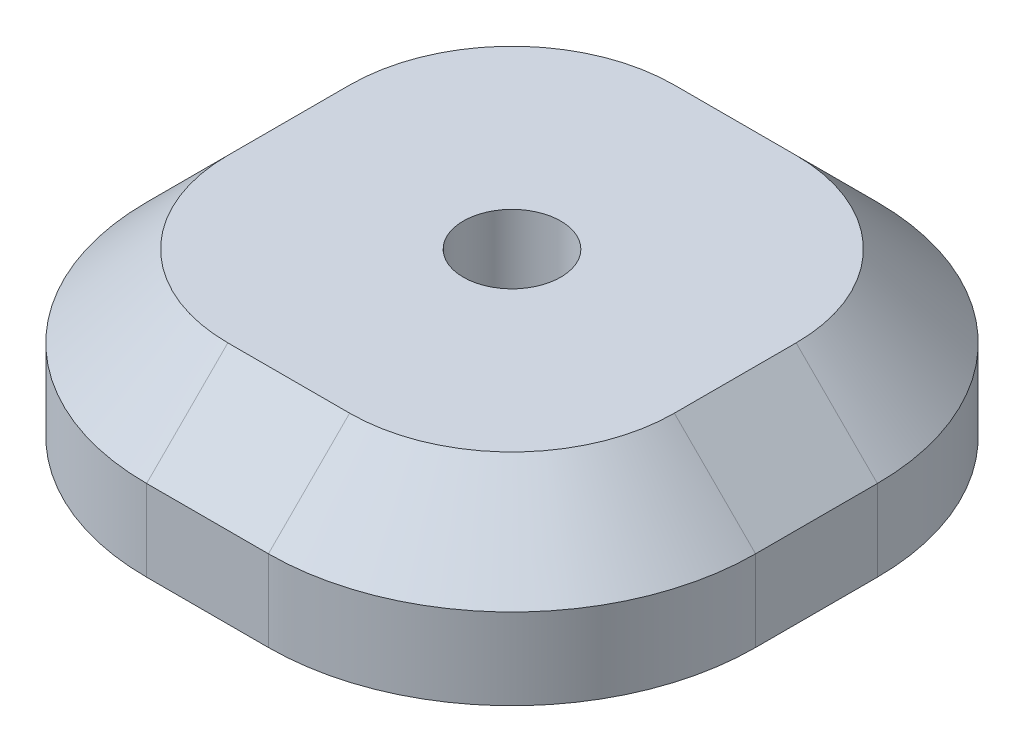
ISO-10303-21;
HEADER;
FILE_DESCRIPTION(('STEP AP214'),'2;1');
FILE_NAME('part.step','',(''),(''),'','','');
FILE_SCHEMA(('AUTOMOTIVE_DESIGN { 1 0 10303 214 1 1 1 1 }'));
ENDSEC;
DATA;
#1=APPLICATION_CONTEXT('core data for automotive mechanical design processes');
#2=APPLICATION_PROTOCOL_DEFINITION('international standard','automotive_design',2000,#1);
#3=PRODUCT_CONTEXT('',#1,'mechanical');
#4=PRODUCT('Part','Part','',(#3));
#5=PRODUCT_RELATED_PRODUCT_CATEGORY('part','',(#4));
#6=PRODUCT_DEFINITION_FORMATION('','',#4);
#7=PRODUCT_DEFINITION_CONTEXT('part definition',#1,'design');
#8=PRODUCT_DEFINITION('design','',#6,#7);
#9=PRODUCT_DEFINITION_SHAPE('','',#8);
#10=(LENGTH_UNIT() NAMED_UNIT(*) SI_UNIT(.MILLI.,.METRE.));
#11=(NAMED_UNIT(*) PLANE_ANGLE_UNIT() SI_UNIT($,.RADIAN.));
#12=(NAMED_UNIT(*) SI_UNIT($,.STERADIAN.) SOLID_ANGLE_UNIT());
#13=UNCERTAINTY_MEASURE_WITH_UNIT(LENGTH_MEASURE(1.E-05),#10,'distance_accuracy_value','');
#14=(GEOMETRIC_REPRESENTATION_CONTEXT(3) GLOBAL_UNCERTAINTY_ASSIGNED_CONTEXT((#13)) GLOBAL_UNIT_ASSIGNED_CONTEXT((#10,
#11,#12)) REPRESENTATION_CONTEXT('',''));
#15=CARTESIAN_POINT('',(0.,0.,0.));
#16=DIRECTION('',(0.,0.,1.));
#17=DIRECTION('',(1.,0.,0.));
#18=AXIS2_PLACEMENT_3D('',#15,#16,#17);
#19=CARTESIAN_POINT('',(37.5,20.,37.5));
#20=DIRECTION('',(-1.,0.,0.));
#21=DIRECTION('',(0.,0.,1.));
#22=AXIS2_PLACEMENT_3D('',#19,#20,#21);
#23=PLANE('',#22);
#24=DIRECTION('',(0.,-1.,0.));
#25=VECTOR('',#24,1.);
#26=CARTESIAN_POINT('',(37.5,20.,-7.5));
#27=LINE('',#26,#25);
#28=CARTESIAN_POINT('',(37.5,0.,-7.5));
#29=VERTEX_POINT('',#28);
#30=CARTESIAN_POINT('',(37.5,9.99999999999995,-7.5));
#31=VERTEX_POINT('',#30);
#32=EDGE_CURVE('E220',#29,#31,#27,.F.);
#33=ORIENTED_EDGE('',*,*,#32,.T.);
#34=DIRECTION('',(0.,0.,1.));
#35=VECTOR('',#34,1.);
#36=CARTESIAN_POINT('',(37.5,9.99999999999995,37.5));
#37=LINE('',#36,#35);
#38=CARTESIAN_POINT('',(37.5,9.99999999999995,7.5));
#39=VERTEX_POINT('',#38);
#40=EDGE_CURVE('E247',#31,#39,#37,.T.);
#41=ORIENTED_EDGE('',*,*,#40,.T.);
#42=DIRECTION('',(0.,-1.,0.));
#43=VECTOR('',#42,1.);
#44=CARTESIAN_POINT('',(37.5,20.,7.5));
#45=LINE('',#44,#43);
#46=CARTESIAN_POINT('',(37.5,0.,7.5));
#47=VERTEX_POINT('',#46);
#48=EDGE_CURVE('E214',#39,#47,#45,.T.);
#49=ORIENTED_EDGE('',*,*,#48,.T.);
#50=DIRECTION('',(0.,0.,-1.));
#51=VECTOR('',#50,1.);
#52=CARTESIAN_POINT('',(37.5,0.,37.5));
#53=LINE('',#52,#51);
#54=EDGE_CURVE('E183',#47,#29,#53,.T.);
#55=ORIENTED_EDGE('',*,*,#54,.T.);
#56=EDGE_LOOP('',(#33,#41,#49,#55));
#57=FACE_BOUND('',#56,.T.);
#58=ADVANCED_FACE('F41',(#57),#23,.F.);
#59=CARTESIAN_POINT('',(-37.5,20.,-37.5));
#60=DIRECTION('',(0.,0.,1.));
#61=DIRECTION('',(1.,0.,0.));
#62=AXIS2_PLACEMENT_3D('',#59,#60,#61);
#63=PLANE('',#62);
#64=DIRECTION('',(0.,-1.,0.));
#65=VECTOR('',#64,1.);
#66=CARTESIAN_POINT('',(-7.49999999999999,20.,-37.5));
#67=LINE('',#66,#65);
#68=CARTESIAN_POINT('',(-7.49999999999999,0.,-37.5));
#69=VERTEX_POINT('',#68);
#70=CARTESIAN_POINT('',(-7.49999999999999,9.99999999999995,-37.5));
#71=VERTEX_POINT('',#70);
#72=EDGE_CURVE('E215',#69,#71,#67,.F.);
#73=ORIENTED_EDGE('',*,*,#72,.T.);
#74=DIRECTION('',(1.,0.,0.));
#75=VECTOR('',#74,1.);
#76=CARTESIAN_POINT('',(-37.5,9.99999999999995,-37.5));
#77=LINE('',#76,#75);
#78=CARTESIAN_POINT('',(7.50000000000001,9.99999999999995,-37.5));
#79=VERTEX_POINT('',#78);
#80=EDGE_CURVE('E243',#71,#79,#77,.T.);
#81=ORIENTED_EDGE('',*,*,#80,.T.);
#82=DIRECTION('',(0.,-1.,0.));
#83=VECTOR('',#82,1.);
#84=CARTESIAN_POINT('',(7.50000000000001,20.,-37.5));
#85=LINE('',#84,#83);
#86=CARTESIAN_POINT('',(7.50000000000001,0.,-37.5));
#87=VERTEX_POINT('',#86);
#88=EDGE_CURVE('E209',#79,#87,#85,.T.);
#89=ORIENTED_EDGE('',*,*,#88,.T.);
#90=DIRECTION('',(-1.,0.,0.));
#91=VECTOR('',#90,1.);
#92=CARTESIAN_POINT('',(-37.5,0.,-37.5));
#93=LINE('',#92,#91);
#94=EDGE_CURVE('E186',#87,#69,#93,.T.);
#95=ORIENTED_EDGE('',*,*,#94,.T.);
#96=EDGE_LOOP('',(#73,#81,#89,#95));
#97=FACE_BOUND('',#96,.T.);
#98=ADVANCED_FACE('F317',(#97),#63,.F.);
#99=CARTESIAN_POINT('',(-37.5,20.,37.5));
#100=DIRECTION('',(1.,0.,0.));
#101=DIRECTION('',(0.,0.,-1.));
#102=AXIS2_PLACEMENT_3D('',#99,#100,#101);
#103=PLANE('',#102);
#104=DIRECTION('',(0.,-1.,0.));
#105=VECTOR('',#104,1.);
#106=CARTESIAN_POINT('',(-37.5,20.,7.5));
#107=LINE('',#106,#105);
#108=CARTESIAN_POINT('',(-37.5,0.,7.5));
#109=VERTEX_POINT('',#108);
#110=CARTESIAN_POINT('',(-37.5,9.99999999999995,7.5));
#111=VERTEX_POINT('',#110);
#112=EDGE_CURVE('E197',#109,#111,#107,.F.);
#113=ORIENTED_EDGE('',*,*,#112,.T.);
#114=DIRECTION('',(0.,0.,-1.));
#115=VECTOR('',#114,1.);
#116=CARTESIAN_POINT('',(-37.5,9.99999999999995,37.5));
#117=LINE('',#116,#115);
#118=CARTESIAN_POINT('',(-37.5,9.99999999999995,-7.5));
#119=VERTEX_POINT('',#118);
#120=EDGE_CURVE('E246',#111,#119,#117,.T.);
#121=ORIENTED_EDGE('',*,*,#120,.T.);
#122=DIRECTION('',(0.,-1.,0.));
#123=VECTOR('',#122,1.);
#124=CARTESIAN_POINT('',(-37.5,20.,-7.5));
#125=LINE('',#124,#123);
#126=CARTESIAN_POINT('',(-37.5,0.,-7.5));
#127=VERTEX_POINT('',#126);
#128=EDGE_CURVE('E199',#119,#127,#125,.T.);
#129=ORIENTED_EDGE('',*,*,#128,.T.);
#130=DIRECTION('',(0.,0.,1.));
#131=VECTOR('',#130,1.);
#132=CARTESIAN_POINT('',(-37.5,0.,37.5));
#133=LINE('',#132,#131);
#134=EDGE_CURVE('E193',#127,#109,#133,.T.);
#135=ORIENTED_EDGE('',*,*,#134,.T.);
#136=EDGE_LOOP('',(#113,#121,#129,#135));
#137=FACE_BOUND('',#136,.T.);
#138=ADVANCED_FACE('F292',(#137),#103,.F.);
#139=CARTESIAN_POINT('',(-37.5,20.,37.5));
#140=DIRECTION('',(0.,0.,-1.));
#141=DIRECTION('',(-1.,0.,0.));
#142=AXIS2_PLACEMENT_3D('',#139,#140,#141);
#143=PLANE('',#142);
#144=DIRECTION('',(0.,-1.,0.));
#145=VECTOR('',#144,1.);
#146=CARTESIAN_POINT('',(7.50000000000001,20.,37.5));
#147=LINE('',#146,#145);
#148=CARTESIAN_POINT('',(7.50000000000001,0.,37.5));
#149=VERTEX_POINT('',#148);
#150=CARTESIAN_POINT('',(7.50000000000001,9.99999999999995,37.5));
#151=VERTEX_POINT('',#150);
#152=EDGE_CURVE('E225',#149,#151,#147,.F.);
#153=ORIENTED_EDGE('',*,*,#152,.T.);
#154=DIRECTION('',(-1.,0.,0.));
#155=VECTOR('',#154,1.);
#156=CARTESIAN_POINT('',(-37.5,9.99999999999995,37.5));
#157=LINE('',#156,#155);
#158=CARTESIAN_POINT('',(-7.49999999999999,9.99999999999995,37.5));
#159=VERTEX_POINT('',#158);
#160=EDGE_CURVE('E11',#151,#159,#157,.T.);
#161=ORIENTED_EDGE('',*,*,#160,.T.);
#162=DIRECTION('',(0.,-1.,0.));
#163=VECTOR('',#162,1.);
#164=CARTESIAN_POINT('',(-7.49999999999999,20.,37.5));
#165=LINE('',#164,#163);
#166=CARTESIAN_POINT('',(-7.49999999999999,0.,37.5));
#167=VERTEX_POINT('',#166);
#168=EDGE_CURVE('E219',#159,#167,#165,.T.);
#169=ORIENTED_EDGE('',*,*,#168,.T.);
#170=DIRECTION('',(1.,0.,0.));
#171=VECTOR('',#170,1.);
#172=CARTESIAN_POINT('',(-37.5,0.,37.5));
#173=LINE('',#172,#171);
#174=EDGE_CURVE('E194',#167,#149,#173,.T.);
#175=ORIENTED_EDGE('',*,*,#174,.T.);
#176=EDGE_LOOP('',(#153,#161,#169,#175));
#177=FACE_BOUND('',#176,.T.);
#178=ADVANCED_FACE('F303',(#177),#143,.F.);
#179=CARTESIAN_POINT('',(0.,20.,0.));
#180=DIRECTION('',(0.,-1.,0.));
#181=DIRECTION('',(0.,0.,-1.));
#182=AXIS2_PLACEMENT_3D('',#179,#180,#181);
#183=PLANE('',#182);
#184=CARTESIAN_POINT('',(0.,20.,0.));
#185=DIRECTION('',(0.,1.,0.));
#186=DIRECTION('',(0.,0.,1.));
#187=AXIS2_PLACEMENT_3D('',#184,#185,#186);
#188=CIRCLE('',#187,5.99999999999999);
#189=CARTESIAN_POINT('',(0.,20.,5.99999999999999));
#190=VERTEX_POINT('',#189);
#191=EDGE_CURVE('E176',#190,#190,#188,.T.);
#192=ORIENTED_EDGE('',*,*,#191,.F.);
#193=EDGE_LOOP('',(#192));
#194=FACE_BOUND('',#193,.T.);
#195=CARTESIAN_POINT('',(7.50000000000001,20.,-7.5));
#196=DIRECTION('',(0.,-1.,0.));
#197=DIRECTION('',(0.,0.,-1.));
#198=AXIS2_PLACEMENT_3D('',#195,#196,#197);
#199=CIRCLE('',#198,20.);
#200=CARTESIAN_POINT('',(27.5,20.,-7.5));
#201=VERTEX_POINT('',#200);
#202=CARTESIAN_POINT('',(7.50000000000001,20.,-27.5));
#203=VERTEX_POINT('',#202);
#204=EDGE_CURVE('E234',#201,#203,#199,.F.);
#205=ORIENTED_EDGE('',*,*,#204,.T.);
#206=DIRECTION('',(-1.,0.,0.));
#207=VECTOR('',#206,1.);
#208=CARTESIAN_POINT('',(0.,20.,-27.5));
#209=LINE('',#208,#207);
#210=CARTESIAN_POINT('',(-7.49999999999999,20.,-27.5));
#211=VERTEX_POINT('',#210);
#212=EDGE_CURVE('E236',#203,#211,#209,.T.);
#213=ORIENTED_EDGE('',*,*,#212,.T.);
#214=CARTESIAN_POINT('',(-7.49999999999999,20.,-7.5));
#215=DIRECTION('',(0.,-1.,0.));
#216=DIRECTION('',(0.,0.,-1.));
#217=AXIS2_PLACEMENT_3D('',#214,#215,#216);
#218=CIRCLE('',#217,20.);
#219=CARTESIAN_POINT('',(-27.5,20.,-7.5));
#220=VERTEX_POINT('',#219);
#221=EDGE_CURVE('E237',#211,#220,#218,.F.);
#222=ORIENTED_EDGE('',*,*,#221,.T.);
#223=DIRECTION('',(0.,0.,1.));
#224=VECTOR('',#223,1.);
#225=CARTESIAN_POINT('',(-27.5,20.,0.));
#226=LINE('',#225,#224);
#227=CARTESIAN_POINT('',(-27.5,20.,7.5));
#228=VERTEX_POINT('',#227);
#229=EDGE_CURVE('E235',#220,#228,#226,.T.);
#230=ORIENTED_EDGE('',*,*,#229,.T.);
#231=CARTESIAN_POINT('',(-7.49999999999999,20.,7.5));
#232=DIRECTION('',(0.,-1.,0.));
#233=DIRECTION('',(0.,0.,-1.));
#234=AXIS2_PLACEMENT_3D('',#231,#232,#233);
#235=CIRCLE('',#234,20.);
#236=CARTESIAN_POINT('',(-7.49999999999999,20.,27.5));
#237=VERTEX_POINT('',#236);
#238=EDGE_CURVE('E226',#228,#237,#235,.F.);
#239=ORIENTED_EDGE('',*,*,#238,.T.);
#240=DIRECTION('',(1.,0.,0.));
#241=VECTOR('',#240,1.);
#242=CARTESIAN_POINT('',(0.,20.,27.5));
#243=LINE('',#242,#241);
#244=CARTESIAN_POINT('',(7.50000000000001,20.,27.5));
#245=VERTEX_POINT('',#244);
#246=EDGE_CURVE('E221',#237,#245,#243,.T.);
#247=ORIENTED_EDGE('',*,*,#246,.T.);
#248=CARTESIAN_POINT('',(7.50000000000001,20.,7.5));
#249=DIRECTION('',(0.,-1.,0.));
#250=DIRECTION('',(0.,0.,-1.));
#251=AXIS2_PLACEMENT_3D('',#248,#249,#250);
#252=CIRCLE('',#251,20.);
#253=CARTESIAN_POINT('',(27.5,20.,7.5));
#254=VERTEX_POINT('',#253);
#255=EDGE_CURVE('E228',#245,#254,#252,.F.);
#256=ORIENTED_EDGE('',*,*,#255,.T.);
#257=DIRECTION('',(0.,0.,-1.));
#258=VECTOR('',#257,1.);
#259=CARTESIAN_POINT('',(27.5,20.,0.));
#260=LINE('',#259,#258);
#261=EDGE_CURVE('E229',#254,#201,#260,.T.);
#262=ORIENTED_EDGE('',*,*,#261,.T.);
#263=EDGE_LOOP('',(#205,#213,#222,#230,#239,#247,#256,#262));
#264=FACE_BOUND('',#263,.T.);
#265=ADVANCED_FACE('F332',(#194,#264),#183,.F.);
#266=CARTESIAN_POINT('',(0.,0.,0.));
#267=DIRECTION('',(0.,-1.,0.));
#268=DIRECTION('',(0.,0.,-1.));
#269=AXIS2_PLACEMENT_3D('',#266,#267,#268);
#270=PLANE('',#269);
#271=CARTESIAN_POINT('',(-12.5,0.,12.5));
#272=DIRECTION('',(0.,-1.,0.));
#273=DIRECTION('',(0.,0.,-1.));
#274=AXIS2_PLACEMENT_3D('',#271,#272,#273);
#275=CIRCLE('',#274,5.99999999999999);
#276=CARTESIAN_POINT('',(-12.5,0.,6.50000000000001));
#277=VERTEX_POINT('',#276);
#278=EDGE_CURVE('E156',#277,#277,#275,.T.);
#279=ORIENTED_EDGE('',*,*,#278,.F.);
#280=EDGE_LOOP('',(#279));
#281=FACE_BOUND('',#280,.T.);
#282=CARTESIAN_POINT('',(12.5,0.,12.5));
#283=DIRECTION('',(0.,-1.,0.));
#284=DIRECTION('',(0.,0.,-1.));
#285=AXIS2_PLACEMENT_3D('',#282,#283,#284);
#286=CIRCLE('',#285,5.99999999999999);
#287=CARTESIAN_POINT('',(12.5,0.,6.50000000000001));
#288=VERTEX_POINT('',#287);
#289=EDGE_CURVE('E154',#288,#288,#286,.T.);
#290=ORIENTED_EDGE('',*,*,#289,.F.);
#291=EDGE_LOOP('',(#290));
#292=FACE_BOUND('',#291,.T.);
#293=CARTESIAN_POINT('',(12.5,0.,-12.5));
#294=DIRECTION('',(0.,-1.,0.));
#295=DIRECTION('',(0.,0.,-1.));
#296=AXIS2_PLACEMENT_3D('',#293,#294,#295);
#297=CIRCLE('',#296,5.99999999999999);
#298=CARTESIAN_POINT('',(12.5,0.,-18.5));
#299=VERTEX_POINT('',#298);
#300=EDGE_CURVE('E167',#299,#299,#297,.T.);
#301=ORIENTED_EDGE('',*,*,#300,.F.);
#302=EDGE_LOOP('',(#301));
#303=FACE_BOUND('',#302,.T.);
#304=CARTESIAN_POINT('',(-12.5,0.,-12.5));
#305=DIRECTION('',(0.,-1.,0.));
#306=DIRECTION('',(0.,0.,-1.));
#307=AXIS2_PLACEMENT_3D('',#304,#305,#306);
#308=CIRCLE('',#307,5.99999999999999);
#309=CARTESIAN_POINT('',(-12.5,0.,-18.5));
#310=VERTEX_POINT('',#309);
#311=EDGE_CURVE('E175',#310,#310,#308,.T.);
#312=ORIENTED_EDGE('',*,*,#311,.F.);
#313=EDGE_LOOP('',(#312));
#314=FACE_BOUND('',#313,.T.);
#315=ORIENTED_EDGE('',*,*,#134,.F.);
#316=CARTESIAN_POINT('',(-7.49999999999999,0.,-7.5));
#317=DIRECTION('',(0.,-1.,0.));
#318=DIRECTION('',(0.,0.,-1.));
#319=AXIS2_PLACEMENT_3D('',#316,#317,#318);
#320=CIRCLE('',#319,30.);
#321=EDGE_CURVE('E208',#127,#69,#320,.T.);
#322=ORIENTED_EDGE('',*,*,#321,.T.);
#323=ORIENTED_EDGE('',*,*,#94,.F.);
#324=CARTESIAN_POINT('',(7.50000000000001,0.,-7.5));
#325=DIRECTION('',(0.,-1.,0.));
#326=DIRECTION('',(0.,0.,-1.));
#327=AXIS2_PLACEMENT_3D('',#324,#325,#326);
#328=CIRCLE('',#327,30.);
#329=EDGE_CURVE('E206',#87,#29,#328,.T.);
#330=ORIENTED_EDGE('',*,*,#329,.T.);
#331=ORIENTED_EDGE('',*,*,#54,.F.);
#332=CARTESIAN_POINT('',(7.50000000000001,0.,7.5));
#333=DIRECTION('',(0.,-1.,0.));
#334=DIRECTION('',(0.,0.,-1.));
#335=AXIS2_PLACEMENT_3D('',#332,#333,#334);
#336=CIRCLE('',#335,30.);
#337=EDGE_CURVE('E204',#47,#149,#336,.T.);
#338=ORIENTED_EDGE('',*,*,#337,.T.);
#339=ORIENTED_EDGE('',*,*,#174,.F.);
#340=CARTESIAN_POINT('',(-7.49999999999999,0.,7.5));
#341=DIRECTION('',(0.,-1.,0.));
#342=DIRECTION('',(0.,0.,-1.));
#343=AXIS2_PLACEMENT_3D('',#340,#341,#342);
#344=CIRCLE('',#343,30.);
#345=EDGE_CURVE('E205',#167,#109,#344,.T.);
#346=ORIENTED_EDGE('',*,*,#345,.T.);
#347=EDGE_LOOP('',(#315,#322,#323,#330,#331,#338,#339,#346));
#348=FACE_BOUND('',#347,.T.);
#349=ADVANCED_FACE('F298',(#281,#292,#303,#314,#348),#270,.T.);
#350=CARTESIAN_POINT('',(-7.49999999999999,20.,-7.5));
#351=DIRECTION('',(0.,-1.,0.));
#352=DIRECTION('',(0.,0.,-1.));
#353=AXIS2_PLACEMENT_3D('',#350,#351,#352);
#354=CYLINDRICAL_SURFACE('',#353,30.);
#355=ORIENTED_EDGE('',*,*,#128,.F.);
#356=CARTESIAN_POINT('',(-7.49999999999999,9.99999999999995,-7.5));
#357=DIRECTION('',(0.,-1.,0.));
#358=DIRECTION('',(0.,0.,-1.));
#359=AXIS2_PLACEMENT_3D('',#356,#357,#358);
#360=CIRCLE('',#359,30.);
#361=EDGE_CURVE('E242',#119,#71,#360,.T.);
#362=ORIENTED_EDGE('',*,*,#361,.T.);
#363=ORIENTED_EDGE('',*,*,#72,.F.);
#364=ORIENTED_EDGE('',*,*,#321,.F.);
#365=EDGE_LOOP('',(#355,#362,#363,#364));
#366=FACE_BOUND('',#365,.T.);
#367=ADVANCED_FACE('F352',(#366),#354,.T.);
#368=CARTESIAN_POINT('',(7.50000000000001,20.,-7.5));
#369=DIRECTION('',(0.,-1.,0.));
#370=DIRECTION('',(0.,0.,-1.));
#371=AXIS2_PLACEMENT_3D('',#368,#369,#370);
#372=CYLINDRICAL_SURFACE('',#371,30.);
#373=ORIENTED_EDGE('',*,*,#88,.F.);
#374=CARTESIAN_POINT('',(7.50000000000001,9.99999999999995,-7.5));
#375=DIRECTION('',(0.,-1.,0.));
#376=DIRECTION('',(0.,0.,-1.));
#377=AXIS2_PLACEMENT_3D('',#374,#375,#376);
#378=CIRCLE('',#377,30.);
#379=EDGE_CURVE('E248',#79,#31,#378,.T.);
#380=ORIENTED_EDGE('',*,*,#379,.T.);
#381=ORIENTED_EDGE('',*,*,#32,.F.);
#382=ORIENTED_EDGE('',*,*,#329,.F.);
#383=EDGE_LOOP('',(#373,#380,#381,#382));
#384=FACE_BOUND('',#383,.T.);
#385=ADVANCED_FACE('F310',(#384),#372,.T.);
#386=CARTESIAN_POINT('',(7.50000000000001,20.,7.5));
#387=DIRECTION('',(0.,-1.,0.));
#388=DIRECTION('',(0.,0.,-1.));
#389=AXIS2_PLACEMENT_3D('',#386,#387,#388);
#390=CYLINDRICAL_SURFACE('',#389,30.);
#391=ORIENTED_EDGE('',*,*,#48,.F.);
#392=CARTESIAN_POINT('',(7.50000000000001,9.99999999999995,7.5));
#393=DIRECTION('',(0.,-1.,0.));
#394=DIRECTION('',(0.,0.,-1.));
#395=AXIS2_PLACEMENT_3D('',#392,#393,#394);
#396=CIRCLE('',#395,30.);
#397=EDGE_CURVE('E51',#39,#151,#396,.T.);
#398=ORIENTED_EDGE('',*,*,#397,.T.);
#399=ORIENTED_EDGE('',*,*,#152,.F.);
#400=ORIENTED_EDGE('',*,*,#337,.F.);
#401=EDGE_LOOP('',(#391,#398,#399,#400));
#402=FACE_BOUND('',#401,.T.);
#403=ADVANCED_FACE('F305',(#402),#390,.T.);
#404=CARTESIAN_POINT('',(-7.49999999999999,20.,7.5));
#405=DIRECTION('',(0.,-1.,0.));
#406=DIRECTION('',(0.,0.,-1.));
#407=AXIS2_PLACEMENT_3D('',#404,#405,#406);
#408=CYLINDRICAL_SURFACE('',#407,30.);
#409=ORIENTED_EDGE('',*,*,#168,.F.);
#410=CARTESIAN_POINT('',(-7.49999999999999,9.99999999999995,7.5));
#411=DIRECTION('',(0.,-1.,0.));
#412=DIRECTION('',(0.,0.,-1.));
#413=AXIS2_PLACEMENT_3D('',#410,#411,#412);
#414=CIRCLE('',#413,30.);
#415=EDGE_CURVE('E252',#159,#111,#414,.T.);
#416=ORIENTED_EDGE('',*,*,#415,.T.);
#417=ORIENTED_EDGE('',*,*,#112,.F.);
#418=ORIENTED_EDGE('',*,*,#345,.F.);
#419=EDGE_LOOP('',(#409,#416,#417,#418));
#420=FACE_BOUND('',#419,.T.);
#421=ADVANCED_FACE('F286',(#420),#408,.T.);
#422=CARTESIAN_POINT('',(0.,20.,27.5));
#423=DIRECTION('',(0.,-0.707106781186546,-0.707106781186549));
#424=DIRECTION('',(1.,0.,0.));
#425=AXIS2_PLACEMENT_3D('',#422,#423,#424);
#426=PLANE('',#425);
#427=DIRECTION('',(0.,0.707106781186549,-0.707106781186546));
#428=VECTOR('',#427,1.);
#429=CARTESIAN_POINT('',(-7.49999999999999,9.99999999999995,37.5));
#430=LINE('',#429,#428);
#431=EDGE_CURVE('E267',#159,#237,#430,.T.);
#432=ORIENTED_EDGE('',*,*,#431,.F.);
#433=ORIENTED_EDGE('',*,*,#160,.F.);
#434=DIRECTION('',(0.,-0.707106781186549,0.707106781186546));
#435=VECTOR('',#434,1.);
#436=CARTESIAN_POINT('',(7.50000000000001,20.,27.5));
#437=LINE('',#436,#435);
#438=EDGE_CURVE('E46',#245,#151,#437,.T.);
#439=ORIENTED_EDGE('',*,*,#438,.F.);
#440=ORIENTED_EDGE('',*,*,#246,.F.);
#441=EDGE_LOOP('',(#432,#433,#439,#440));
#442=FACE_BOUND('',#441,.T.);
#443=ADVANCED_FACE('F42',(#442),#426,.F.);
#444=CARTESIAN_POINT('',(7.50000000000001,20.,7.5));
#445=DIRECTION('',(0.,-1.,0.));
#446=DIRECTION('',(0.,0.,-1.));
#447=AXIS2_PLACEMENT_3D('',#444,#445,#446);
#448=CONICAL_SURFACE('',#447,20.,0.785398163397446);
#449=ORIENTED_EDGE('',*,*,#438,.T.);
#450=ORIENTED_EDGE('',*,*,#397,.F.);
#451=DIRECTION('',(0.707106781186546,-0.707106781186549,0.));
#452=VECTOR('',#451,1.);
#453=CARTESIAN_POINT('',(27.5,20.,7.5));
#454=LINE('',#453,#452);
#455=EDGE_CURVE('E270',#254,#39,#454,.T.);
#456=ORIENTED_EDGE('',*,*,#455,.F.);
#457=ORIENTED_EDGE('',*,*,#255,.F.);
#458=EDGE_LOOP('',(#449,#450,#456,#457));
#459=FACE_BOUND('',#458,.T.);
#460=ADVANCED_FACE('F276',(#459),#448,.T.);
#461=CARTESIAN_POINT('',(-7.49999999999999,20.,7.5));
#462=DIRECTION('',(0.,-1.,0.));
#463=DIRECTION('',(0.,0.,-1.));
#464=AXIS2_PLACEMENT_3D('',#461,#462,#463);
#465=CONICAL_SURFACE('',#464,20.,0.785398163397446);
#466=ORIENTED_EDGE('',*,*,#431,.T.);
#467=ORIENTED_EDGE('',*,*,#238,.F.);
#468=DIRECTION('',(0.707106781186546,0.707106781186549,0.));
#469=VECTOR('',#468,1.);
#470=CARTESIAN_POINT('',(-37.5,9.99999999999995,7.5));
#471=LINE('',#470,#469);
#472=EDGE_CURVE('E262',#111,#228,#471,.T.);
#473=ORIENTED_EDGE('',*,*,#472,.F.);
#474=ORIENTED_EDGE('',*,*,#415,.F.);
#475=EDGE_LOOP('',(#466,#467,#473,#474));
#476=FACE_BOUND('',#475,.T.);
#477=ADVANCED_FACE('F282',(#476),#465,.T.);
#478=CARTESIAN_POINT('',(27.5,20.,0.));
#479=DIRECTION('',(-0.707106781186549,-0.707106781186546,0.));
#480=DIRECTION('',(0.,0.,-1.));
#481=AXIS2_PLACEMENT_3D('',#478,#479,#480);
#482=PLANE('',#481);
#483=ORIENTED_EDGE('',*,*,#455,.T.);
#484=ORIENTED_EDGE('',*,*,#40,.F.);
#485=DIRECTION('',(0.707106781186546,-0.707106781186549,0.));
#486=VECTOR('',#485,1.);
#487=CARTESIAN_POINT('',(27.5,20.,-7.5));
#488=LINE('',#487,#486);
#489=EDGE_CURVE('E261',#201,#31,#488,.T.);
#490=ORIENTED_EDGE('',*,*,#489,.F.);
#491=ORIENTED_EDGE('',*,*,#261,.F.);
#492=EDGE_LOOP('',(#483,#484,#490,#491));
#493=FACE_BOUND('',#492,.T.);
#494=ADVANCED_FACE('F331',(#493),#482,.F.);
#495=CARTESIAN_POINT('',(-27.5,20.,0.));
#496=DIRECTION('',(0.707106781186549,-0.707106781186546,0.));
#497=DIRECTION('',(0.,0.,1.));
#498=AXIS2_PLACEMENT_3D('',#495,#496,#497);
#499=PLANE('',#498);
#500=ORIENTED_EDGE('',*,*,#472,.T.);
#501=ORIENTED_EDGE('',*,*,#229,.F.);
#502=DIRECTION('',(0.707106781186546,0.707106781186549,0.));
#503=VECTOR('',#502,1.);
#504=CARTESIAN_POINT('',(-37.5,9.99999999999995,-7.5));
#505=LINE('',#504,#503);
#506=EDGE_CURVE('E256',#119,#220,#505,.T.);
#507=ORIENTED_EDGE('',*,*,#506,.F.);
#508=ORIENTED_EDGE('',*,*,#120,.F.);
#509=EDGE_LOOP('',(#500,#501,#507,#508));
#510=FACE_BOUND('',#509,.T.);
#511=ADVANCED_FACE('F338',(#510),#499,.F.);
#512=CARTESIAN_POINT('',(7.50000000000001,20.,-7.5));
#513=DIRECTION('',(0.,-1.,0.));
#514=DIRECTION('',(0.,0.,-1.));
#515=AXIS2_PLACEMENT_3D('',#512,#513,#514);
#516=CONICAL_SURFACE('',#515,20.,0.785398163397446);
#517=ORIENTED_EDGE('',*,*,#489,.T.);
#518=ORIENTED_EDGE('',*,*,#379,.F.);
#519=DIRECTION('',(0.,-0.707106781186549,-0.707106781186546));
#520=VECTOR('',#519,1.);
#521=CARTESIAN_POINT('',(7.50000000000001,20.,-27.5));
#522=LINE('',#521,#520);
#523=EDGE_CURVE('E258',#203,#79,#522,.T.);
#524=ORIENTED_EDGE('',*,*,#523,.F.);
#525=ORIENTED_EDGE('',*,*,#204,.F.);
#526=EDGE_LOOP('',(#517,#518,#524,#525));
#527=FACE_BOUND('',#526,.T.);
#528=ADVANCED_FACE('F311',(#527),#516,.T.);
#529=CARTESIAN_POINT('',(-7.49999999999999,20.,-7.5));
#530=DIRECTION('',(0.,-1.,0.));
#531=DIRECTION('',(0.,0.,-1.));
#532=AXIS2_PLACEMENT_3D('',#529,#530,#531);
#533=CONICAL_SURFACE('',#532,20.,0.785398163397446);
#534=ORIENTED_EDGE('',*,*,#506,.T.);
#535=ORIENTED_EDGE('',*,*,#221,.F.);
#536=DIRECTION('',(0.,0.707106781186549,0.707106781186546));
#537=VECTOR('',#536,1.);
#538=CARTESIAN_POINT('',(-7.49999999999999,9.99999999999995,-37.5));
#539=LINE('',#538,#537);
#540=EDGE_CURVE('E184',#71,#211,#539,.T.);
#541=ORIENTED_EDGE('',*,*,#540,.F.);
#542=ORIENTED_EDGE('',*,*,#361,.F.);
#543=EDGE_LOOP('',(#534,#535,#541,#542));
#544=FACE_BOUND('',#543,.T.);
#545=ADVANCED_FACE('F330',(#544),#533,.T.);
#546=CARTESIAN_POINT('',(0.,20.,-27.5));
#547=DIRECTION('',(0.,-0.707106781186546,0.707106781186549));
#548=DIRECTION('',(-1.,0.,0.));
#549=AXIS2_PLACEMENT_3D('',#546,#547,#548);
#550=PLANE('',#549);
#551=ORIENTED_EDGE('',*,*,#523,.T.);
#552=ORIENTED_EDGE('',*,*,#80,.F.);
#553=ORIENTED_EDGE('',*,*,#540,.T.);
#554=ORIENTED_EDGE('',*,*,#212,.F.);
#555=EDGE_LOOP('',(#551,#552,#553,#554));
#556=FACE_BOUND('',#555,.T.);
#557=ADVANCED_FACE('F323',(#556),#550,.F.);
#558=CARTESIAN_POINT('',(0.,10.,0.));
#559=DIRECTION('',(0.,1.,0.));
#560=DIRECTION('',(0.,0.,1.));
#561=AXIS2_PLACEMENT_3D('',#558,#559,#560);
#562=CONICAL_SURFACE('',#561,5.99999999999999,1.02974425867665);
#563=CARTESIAN_POINT('',(0.,6.39483628583465,0.));
#564=VERTEX_POINT('',#563);
#565=VERTEX_LOOP('',#564);
#566=FACE_BOUND('',#565,.T.);
#567=CARTESIAN_POINT('',(0.,10.,0.));
#568=DIRECTION('',(0.,1.,0.));
#569=DIRECTION('',(0.,0.,1.));
#570=AXIS2_PLACEMENT_3D('',#567,#568,#569);
#571=CIRCLE('',#570,5.99999999999999);
#572=CARTESIAN_POINT('',(0.,10.,5.99999999999999));
#573=VERTEX_POINT('',#572);
#574=EDGE_CURVE('E182',#573,#573,#571,.T.);
#575=ORIENTED_EDGE('',*,*,#574,.T.);
#576=EDGE_LOOP('',(#575));
#577=FACE_BOUND('',#576,.T.);
#578=ADVANCED_FACE('F367',(#566,#577),#562,.F.);
#579=CARTESIAN_POINT('',(0.,20.,0.));
#580=DIRECTION('',(0.,1.,0.));
#581=DIRECTION('',(0.,0.,1.));
#582=AXIS2_PLACEMENT_3D('',#579,#580,#581);
#583=CYLINDRICAL_SURFACE('',#582,5.99999999999999);
#584=ORIENTED_EDGE('',*,*,#574,.F.);
#585=EDGE_LOOP('',(#584));
#586=FACE_BOUND('',#585,.T.);
#587=ORIENTED_EDGE('',*,*,#191,.T.);
#588=EDGE_LOOP('',(#587));
#589=FACE_BOUND('',#588,.T.);
#590=ADVANCED_FACE('F504',(#586,#589),#583,.F.);
#591=CARTESIAN_POINT('',(-12.5,9.99999999999999,-12.5));
#592=DIRECTION('',(0.,-1.,0.));
#593=DIRECTION('',(0.,0.,-1.));
#594=AXIS2_PLACEMENT_3D('',#591,#592,#593);
#595=CONICAL_SURFACE('',#594,5.99999999999999,1.02974425867665);
#596=CARTESIAN_POINT('',(-12.5,13.6051637141654,-12.5));
#597=VERTEX_POINT('',#596);
#598=VERTEX_LOOP('',#597);
#599=FACE_BOUND('',#598,.T.);
#600=CARTESIAN_POINT('',(-12.5,9.99999999999999,-12.5));
#601=DIRECTION('',(0.,-1.,0.));
#602=DIRECTION('',(0.,0.,-1.));
#603=AXIS2_PLACEMENT_3D('',#600,#601,#602);
#604=CIRCLE('',#603,5.99999999999999);
#605=CARTESIAN_POINT('',(-12.5,9.99999999999999,-18.5));
#606=VERTEX_POINT('',#605);
#607=EDGE_CURVE('E174',#606,#606,#604,.T.);
#608=ORIENTED_EDGE('',*,*,#607,.T.);
#609=EDGE_LOOP('',(#608));
#610=FACE_BOUND('',#609,.T.);
#611=ADVANCED_FACE('F514',(#599,#610),#595,.F.);
#612=CARTESIAN_POINT('',(-12.5,0.,-12.5));
#613=DIRECTION('',(0.,-1.,0.));
#614=DIRECTION('',(0.,0.,-1.));
#615=AXIS2_PLACEMENT_3D('',#612,#613,#614);
#616=CYLINDRICAL_SURFACE('',#615,5.99999999999999);
#617=ORIENTED_EDGE('',*,*,#607,.F.);
#618=EDGE_LOOP('',(#617));
#619=FACE_BOUND('',#618,.T.);
#620=ORIENTED_EDGE('',*,*,#311,.T.);
#621=EDGE_LOOP('',(#620));
#622=FACE_BOUND('',#621,.T.);
#623=ADVANCED_FACE('F521',(#619,#622),#616,.F.);
#624=CARTESIAN_POINT('',(12.5,9.99999999999999,-12.5));
#625=DIRECTION('',(0.,-1.,0.));
#626=DIRECTION('',(0.,0.,-1.));
#627=AXIS2_PLACEMENT_3D('',#624,#625,#626);
#628=CONICAL_SURFACE('',#627,5.99999999999999,1.02974425867665);
#629=CARTESIAN_POINT('',(12.5,13.6051637141654,-12.5));
#630=VERTEX_POINT('',#629);
#631=VERTEX_LOOP('',#630);
#632=FACE_BOUND('',#631,.T.);
#633=CARTESIAN_POINT('',(12.5,9.99999999999999,-12.5));
#634=DIRECTION('',(0.,-1.,0.));
#635=DIRECTION('',(0.,0.,-1.));
#636=AXIS2_PLACEMENT_3D('',#633,#634,#635);
#637=CIRCLE('',#636,5.99999999999999);
#638=CARTESIAN_POINT('',(12.5,9.99999999999999,-18.5));
#639=VERTEX_POINT('',#638);
#640=EDGE_CURVE('E166',#639,#639,#637,.T.);
#641=ORIENTED_EDGE('',*,*,#640,.T.);
#642=EDGE_LOOP('',(#641));
#643=FACE_BOUND('',#642,.T.);
#644=ADVANCED_FACE('F535',(#632,#643),#628,.F.);
#645=CARTESIAN_POINT('',(12.5,0.,-12.5));
#646=DIRECTION('',(0.,-1.,0.));
#647=DIRECTION('',(0.,0.,-1.));
#648=AXIS2_PLACEMENT_3D('',#645,#646,#647);
#649=CYLINDRICAL_SURFACE('',#648,5.99999999999999);
#650=ORIENTED_EDGE('',*,*,#640,.F.);
#651=EDGE_LOOP('',(#650));
#652=FACE_BOUND('',#651,.T.);
#653=ORIENTED_EDGE('',*,*,#300,.T.);
#654=EDGE_LOOP('',(#653));
#655=FACE_BOUND('',#654,.T.);
#656=ADVANCED_FACE('F541',(#652,#655),#649,.F.);
#657=CARTESIAN_POINT('',(12.5,9.99999999999999,12.5));
#658=DIRECTION('',(0.,-1.,0.));
#659=DIRECTION('',(0.,0.,-1.));
#660=AXIS2_PLACEMENT_3D('',#657,#658,#659);
#661=CONICAL_SURFACE('',#660,5.99999999999999,1.02974425867665);
#662=CARTESIAN_POINT('',(12.5,13.6051637141654,12.5));
#663=VERTEX_POINT('',#662);
#664=VERTEX_LOOP('',#663);
#665=FACE_BOUND('',#664,.T.);
#666=CARTESIAN_POINT('',(12.5,9.99999999999999,12.5));
#667=DIRECTION('',(0.,-1.,0.));
#668=DIRECTION('',(0.,0.,-1.));
#669=AXIS2_PLACEMENT_3D('',#666,#667,#668);
#670=CIRCLE('',#669,5.99999999999999);
#671=CARTESIAN_POINT('',(12.5,9.99999999999999,6.50000000000001));
#672=VERTEX_POINT('',#671);
#673=EDGE_CURVE('E157',#672,#672,#670,.T.);
#674=ORIENTED_EDGE('',*,*,#673,.T.);
#675=EDGE_LOOP('',(#674));
#676=FACE_BOUND('',#675,.T.);
#677=ADVANCED_FACE('F549',(#665,#676),#661,.F.);
#678=CARTESIAN_POINT('',(12.5,0.,12.5));
#679=DIRECTION('',(0.,-1.,0.));
#680=DIRECTION('',(0.,0.,-1.));
#681=AXIS2_PLACEMENT_3D('',#678,#679,#680);
#682=CYLINDRICAL_SURFACE('',#681,5.99999999999999);
#683=ORIENTED_EDGE('',*,*,#673,.F.);
#684=EDGE_LOOP('',(#683));
#685=FACE_BOUND('',#684,.T.);
#686=ORIENTED_EDGE('',*,*,#289,.T.);
#687=EDGE_LOOP('',(#686));
#688=FACE_BOUND('',#687,.T.);
#689=ADVANCED_FACE('F149',(#685,#688),#682,.F.);
#690=CARTESIAN_POINT('',(-12.5,9.99999999999999,12.5));
#691=DIRECTION('',(0.,-1.,0.));
#692=DIRECTION('',(0.,0.,-1.));
#693=AXIS2_PLACEMENT_3D('',#690,#691,#692);
#694=CONICAL_SURFACE('',#693,5.99999999999999,1.02974425867665);
#695=CARTESIAN_POINT('',(-12.5,13.6051637141654,12.5));
#696=VERTEX_POINT('',#695);
#697=VERTEX_LOOP('',#696);
#698=FACE_BOUND('',#697,.T.);
#699=CARTESIAN_POINT('',(-12.5,9.99999999999999,12.5));
#700=DIRECTION('',(0.,-1.,0.));
#701=DIRECTION('',(0.,0.,-1.));
#702=AXIS2_PLACEMENT_3D('',#699,#700,#701);
#703=CIRCLE('',#702,5.99999999999999);
#704=CARTESIAN_POINT('',(-12.5,9.99999999999999,6.50000000000001));
#705=VERTEX_POINT('',#704);
#706=EDGE_CURVE('E153',#705,#705,#703,.T.);
#707=ORIENTED_EDGE('',*,*,#706,.T.);
#708=EDGE_LOOP('',(#707));
#709=FACE_BOUND('',#708,.T.);
#710=ADVANCED_FACE('F144',(#698,#709),#694,.F.);
#711=CARTESIAN_POINT('',(-12.5,0.,12.5));
#712=DIRECTION('',(0.,-1.,0.));
#713=DIRECTION('',(0.,0.,-1.));
#714=AXIS2_PLACEMENT_3D('',#711,#712,#713);
#715=CYLINDRICAL_SURFACE('',#714,5.99999999999999);
#716=ORIENTED_EDGE('',*,*,#706,.F.);
#717=EDGE_LOOP('',(#716));
#718=FACE_BOUND('',#717,.T.);
#719=ORIENTED_EDGE('',*,*,#278,.T.);
#720=EDGE_LOOP('',(#719));
#721=FACE_BOUND('',#720,.T.);
#722=ADVANCED_FACE('F146',(#718,#721),#715,.F.);
#723=CLOSED_SHELL('',(#58,#98,#138,#178,#265,#349,#367,#385,#403,#421,#443,#460,#477,#494,#511,
#528,#545,#557,#578,#590,#611,#623,#644,#656,#677,#689,#710,#722));
#724=MANIFOLD_SOLID_BREP('B2',#723);
#725=ADVANCED_BREP_SHAPE_REPRESENTATION('',(#18,#724),#14);
#726=SHAPE_DEFINITION_REPRESENTATION(#9,#725);
ENDSEC;
END-ISO-10303-21;
